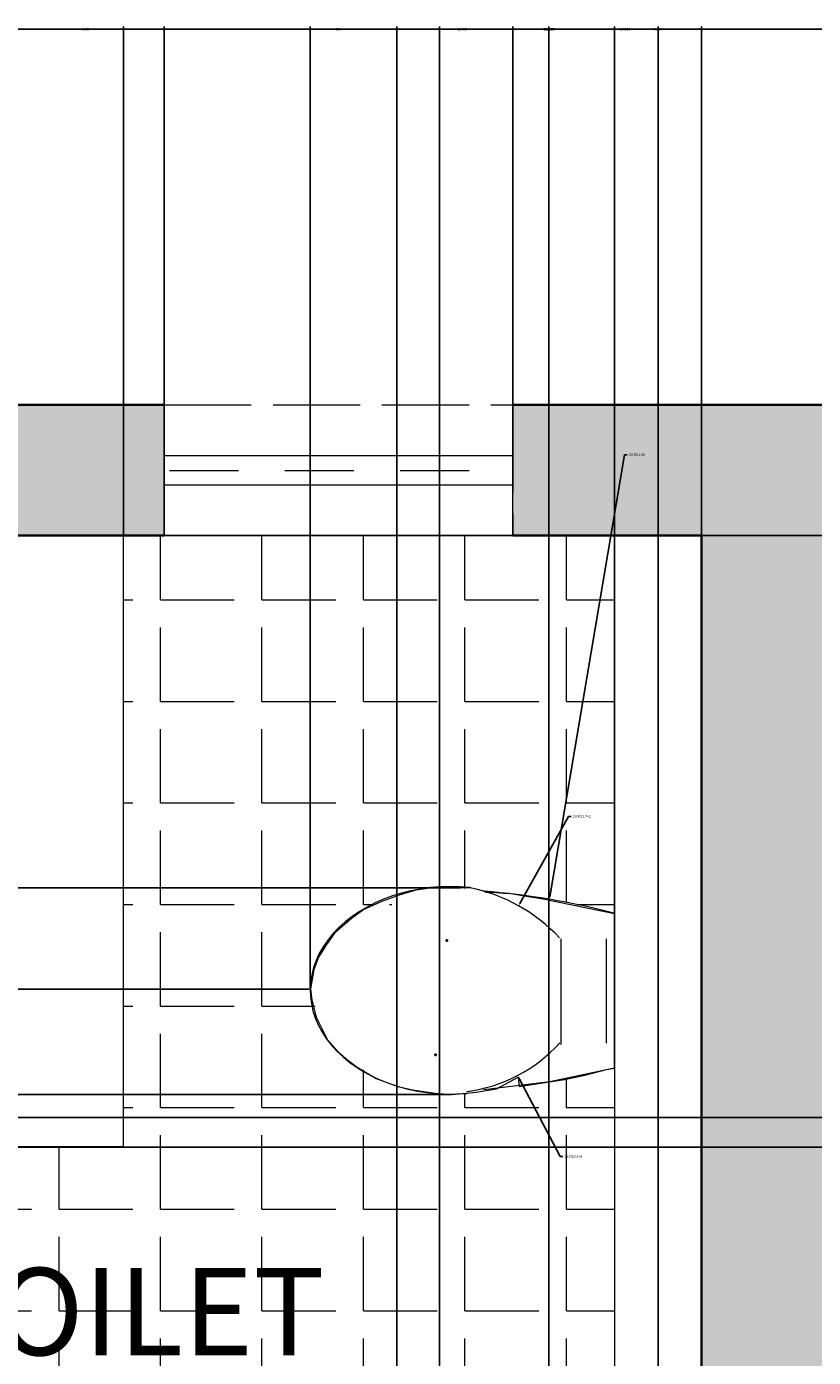
# Model space of a CAD drawing. Units: inches. Extents: x 6 to 575, y 34 to 566.
# Tile 11 of 21: x 151 to 205, y 474 to 566. Entities that reach past the tile are written whole.
import ezdxf

# ---------------------------------------------------------------- set-up
doc = ezdxf.new("R2010")
doc.units = ezdxf.units.IN
doc.linetypes.add('ACAD_ISO02W100', pattern=[15, 12, -3])
for name, color, linetype, lineweight in [('A-ANNO-DIMS', 2, 'Continuous', 18), ('A-AREA-IDEN', 6, 'Continuous', 20), ('A-FLOR-CASE', 2, 'Continuous', 18), ('A-FLOR-FIXT', 9, 'Continuous', 18), ('A-FLOR-PATT', 252, 'Continuous', 9), ('A-GLAZ-HIDN', 4, 'ACAD_ISO02W100', 18), ('A-GLAZ-PATT', 4, 'Continuous', 9), ('A-WALL-PATT', 251, 'Continuous', 9), ('WALLS', 7, 'Continuous', 35), ('WINDOWS', 4, 'Continuous', 20)]:
    doc.layers.add(name, color=color, linetype=linetype, lineweight=lineweight)
doc.styles.add('PDF Arial Narrow', font='txt')
doc.styles.get("Standard").update_dxf_attribs({"font": 'arial.ttf'})
doc.dimstyles.get("Standard").update_dxf_attribs({"dimtxt": 0.18, "dimasz": 0.18, "dimexe": 0.18, "dimexo": 0.0625, "dimgap": 0.09, "dimtad": 0, "dimtih": 1, "dimtoh": 1, "dimdec": 4, "dimzin": 0, "dimdsep": 46, "dimtxsty": 'Standard', "dimcen": 0.09, "dimadec": 0, "dimazin": 0, "dimtfac": 1, "dimtdec": 4, "dimtofl": 0, "dimtmove": 0, "dimatfit": 3, "dimfxl": 1, "dimtolj": 1, "dimtzin": 0, "dimarcsym": 0})

# ---------------------------------------------------------------- blocks, each defined once
blk = doc.blocks.new('*D30')
at = {"layer": 'A-ANNO-DIMS', "color": 0, "lineweight": -2, "transparency": 16777216}
for p, q in [((32.596, 539.801), (6.649, 539.801)), ((6.829, 539.621), (6.829, 299.97)), ((6.829, 59.955), (6.829, 299.606)), ((197.625, 59.775), (6.649, 59.775))]:
    blk.add_line(p, q, dxfattribs=at)
at = {"layer": 'A-ANNO-DIMS', "color": 0, "transparency": 16777216}
for points in [[(6.799, 539.621), (6.859, 539.621), (6.829, 539.801)], [(6.799, 59.955), (6.859, 59.955), (6.829, 59.775)]]:
    blk.add_solid(points, dxfattribs=at)
at = {"layer": 'Defpoints', "color": 0, "transparency": 16777216}
for p in [(32.659, 539.801), (6.829, 59.775), (197.687, 59.775)]:
    blk.add_point(p, dxfattribs=at)
at = {"layer": 'A-ANNO-DIMS', "color": 0, "transparency": 16777216, "insert": (6.829, 299.788), "char_height": 0.18, "attachment_point": 5}
blk.add_mtext('\\A1;480', dxfattribs=at)
blk = doc.blocks.new('*D31')
at = {"layer": 'A-ANNO-DIMS', "color": 0, "lineweight": -2, "transparency": 16777216}
for p, q in [((32.659, 539.863), (32.659, 565.811)), ((160.659, 539.863), (160.659, 565.811)), ((32.839, 565.631), (96.378, 565.631)), ((160.479, 565.631), (96.939, 565.631))]:
    blk.add_line(p, q, dxfattribs=at)
at = {"layer": 'A-ANNO-DIMS', "color": 0, "transparency": 16777216}
for points in [[(32.839, 565.661), (32.839, 565.601), (32.659, 565.631)], [(160.479, 565.661), (160.479, 565.601), (160.659, 565.631)]]:
    blk.add_solid(points, dxfattribs=at)
at = {"layer": 'Defpoints', "color": 0, "transparency": 16777216}
for p in [(160.659, 565.631), (32.659, 539.801), (160.659, 539.801)]:
    blk.add_point(p, dxfattribs=at)
at = {"layer": 'A-ANNO-DIMS', "color": 0, "transparency": 16777216, "insert": (96.659, 565.631), "char_height": 0.18, "attachment_point": 5}
blk.add_mtext('\\A1;128', dxfattribs=at)
blk = doc.blocks.new('*D32')
at = {"layer": 'A-ANNO-DIMS', "color": 0, "lineweight": -2, "transparency": 16777216}
for p, q in [((160.659, 539.863), (160.659, 565.811)), ((184.659, 539.863), (184.659, 565.811)), ((160.839, 565.631), (172.439, 565.631)), ((184.479, 565.631), (172.879, 565.631))]:
    blk.add_line(p, q, dxfattribs=at)
at = {"layer": 'A-ANNO-DIMS', "color": 0, "transparency": 16777216}
for points in [[(160.839, 565.661), (160.839, 565.601), (160.659, 565.631)], [(184.479, 565.661), (184.479, 565.601), (184.659, 565.631)]]:
    blk.add_solid(points, dxfattribs=at)
at = {"layer": 'Defpoints', "color": 0, "transparency": 16777216}
for p in [(184.659, 565.631), (160.659, 539.801), (184.659, 539.801)]:
    blk.add_point(p, dxfattribs=at)
at = {"layer": 'A-ANNO-DIMS', "color": 0, "transparency": 16777216, "insert": (172.659, 565.631), "char_height": 0.18, "attachment_point": 5}
blk.add_mtext('\\A1;24', dxfattribs=at)
blk = doc.blocks.new('*D33')
at = {"layer": 'A-ANNO-DIMS', "color": 0, "lineweight": -2, "transparency": 16777216}
for p, q in [((184.659, 539.863), (184.659, 565.811)), ((272.659, 539.863), (272.659, 565.811)), ((184.839, 565.631), (228.439, 565.631)), ((272.479, 565.631), (228.878, 565.631))]:
    blk.add_line(p, q, dxfattribs=at)
at = {"layer": 'A-ANNO-DIMS', "color": 0, "transparency": 16777216}
for points in [[(184.839, 565.661), (184.839, 565.601), (184.659, 565.631)], [(272.479, 565.661), (272.479, 565.601), (272.659, 565.631)]]:
    blk.add_solid(points, dxfattribs=at)
at = {"layer": 'Defpoints', "color": 0, "transparency": 16777216}
for p in [(272.659, 565.631), (184.659, 539.801), (272.659, 539.801)]:
    blk.add_point(p, dxfattribs=at)
at = {"layer": 'A-ANNO-DIMS', "color": 0, "transparency": 16777216, "insert": (228.659, 565.631), "char_height": 0.18, "attachment_point": 5}
blk.add_mtext('\\A1;88', dxfattribs=at)
blk = doc.blocks.new('*D68')
at = {"layer": 'A-ANNO-DIMS', "color": 0, "lineweight": -2, "transparency": 16777216}
for p, q in [((206.596, 530.801), (6.649, 530.801)), ((6.829, 530.621), (6.829, 509.957)), ((6.829, 488.928), (6.829, 509.593)), ((248.571, 488.748), (6.649, 488.748))]:
    blk.add_line(p, q, dxfattribs=at)
at = {"layer": 'A-ANNO-DIMS', "color": 0, "transparency": 16777216}
for points in [[(6.799, 530.621), (6.859, 530.621), (6.829, 530.801)], [(6.799, 488.928), (6.859, 488.928), (6.829, 488.748)]]:
    blk.add_solid(points, dxfattribs=at)
at = {"layer": 'Defpoints', "color": 0, "transparency": 16777216}
for p in [(206.659, 530.801), (6.829, 488.748), (248.633, 488.748)]:
    blk.add_point(p, dxfattribs=at)
at = {"layer": 'A-ANNO-DIMS', "color": 0, "transparency": 16777216, "insert": (6.829, 509.775), "char_height": 0.18, "attachment_point": 5}
blk.add_mtext('\\A1;42.05', dxfattribs=at)
blk = doc.blocks.new('*D71')
at = {"layer": 'A-ANNO-DIMS', "color": 0, "lineweight": -2, "transparency": 16777216}
for p, q in [((246.62, 490.777), (6.649, 490.777)), ((6.829, 490.597), (6.829, 489.945)), ((6.829, 488.928), (6.829, 489.581)), ((248.571, 488.748), (6.649, 488.748))]:
    blk.add_line(p, q, dxfattribs=at)
at = {"layer": 'A-ANNO-DIMS', "color": 0, "transparency": 16777216}
for points in [[(6.799, 490.597), (6.859, 490.597), (6.829, 490.777)], [(6.799, 488.928), (6.859, 488.928), (6.829, 488.748)]]:
    blk.add_solid(points, dxfattribs=at)
at = {"layer": 'Defpoints', "color": 0, "transparency": 16777216}
for p in [(246.683, 490.777), (6.829, 488.748), (248.633, 488.748)]:
    blk.add_point(p, dxfattribs=at)
at = {"layer": 'A-ANNO-DIMS', "color": 0, "transparency": 16777216, "insert": (6.829, 489.763), "char_height": 0.18, "attachment_point": 5}
blk.add_mtext('\\A1;2.03', dxfattribs=at)
blk = doc.blocks.new('*D109')
at = {"layer": 'A-ANNO-DIMS', "color": 0, "lineweight": -2, "transparency": 16777216}
for p, q in [((112.851, 431.863), (112.851, 565.811)), ((197.659, 431.863), (197.659, 565.811)), ((113.031, 565.631), (154.931, 565.631)), ((197.479, 565.631), (155.579, 565.631))]:
    blk.add_line(p, q, dxfattribs=at)
at = {"layer": 'A-ANNO-DIMS', "color": 0, "transparency": 16777216}
for points in [[(113.031, 565.661), (113.031, 565.601), (112.851, 565.631)], [(197.479, 565.661), (197.479, 565.601), (197.659, 565.631)]]:
    blk.add_solid(points, dxfattribs=at)
at = {"layer": 'Defpoints', "color": 0, "transparency": 16777216}
for p in [(197.659, 565.631), (112.851, 431.801), (197.659, 431.801)]:
    blk.add_point(p, dxfattribs=at)
at = {"layer": 'A-ANNO-DIMS', "color": 0, "transparency": 16777216, "insert": (155.255, 565.631), "char_height": 0.18, "attachment_point": 5}
blk.add_mtext('\\A1;84.8', dxfattribs=at)
blk = doc.blocks.new('*D175')
at = {"layer": 'A-ANNO-DIMS', "color": 0, "lineweight": -2, "transparency": 16777216}
for p, q in [((121.659, 530.863), (121.659, 565.811)), ((157.869, 530.898), (157.869, 565.811)), ((121.839, 565.631), (139.387, 565.631)), ((157.689, 565.631), (140.14, 565.631))]:
    blk.add_line(p, q, dxfattribs=at)
at = {"layer": 'A-ANNO-DIMS', "color": 0, "transparency": 16777216}
for points in [[(121.839, 565.661), (121.839, 565.601), (121.659, 565.631)], [(157.689, 565.661), (157.689, 565.601), (157.869, 565.631)]]:
    blk.add_solid(points, dxfattribs=at)
at = {"layer": 'Defpoints', "color": 0, "transparency": 16777216}
for p in [(157.869, 565.631), (121.659, 530.801), (157.869, 530.836)]:
    blk.add_point(p, dxfattribs=at)
at = {"layer": 'A-ANNO-DIMS', "color": 0, "transparency": 16777216, "insert": (139.764, 565.631), "char_height": 0.18, "attachment_point": 5}
blk.add_mtext('\\A1;36.21', dxfattribs=at)
blk = doc.blocks.new('*D181')
at = {"layer": 'A-ANNO-DIMS', "color": 0, "lineweight": -2, "transparency": 16777216}
for p, q in [((197.596, 530.801), (6.649, 530.801)), ((6.829, 530.621), (6.829, 515.387)), ((6.829, 499.788), (6.829, 515.023)), ((170.657, 499.608), (6.649, 499.608))]:
    blk.add_line(p, q, dxfattribs=at)
at = {"layer": 'A-ANNO-DIMS', "color": 0, "transparency": 16777216}
for points in [[(6.799, 530.621), (6.859, 530.621), (6.829, 530.801)], [(6.799, 499.788), (6.859, 499.788), (6.829, 499.608)]]:
    blk.add_solid(points, dxfattribs=at)
at = {"layer": 'Defpoints', "color": 0, "transparency": 16777216}
for p in [(197.659, 530.801), (6.829, 499.608), (170.719, 499.608)]:
    blk.add_point(p, dxfattribs=at)
at = {"layer": 'A-ANNO-DIMS', "color": 0, "transparency": 16777216, "insert": (6.829, 515.205), "char_height": 0.18, "attachment_point": 5}
blk.add_mtext('\\A1;31.19', dxfattribs=at)
blk = doc.blocks.new('*D182')
at = {"layer": 'A-ANNO-DIMS', "color": 0, "lineweight": -2, "transparency": 16777216}
for p, q in [((170.719, 499.671), (170.719, 565.811)), ((191.651, 504.84), (191.651, 565.811)), ((170.899, 565.631), (180.79, 565.631)), ((191.471, 565.631), (181.581, 565.631))]:
    blk.add_line(p, q, dxfattribs=at)
at = {"layer": 'A-ANNO-DIMS', "color": 0, "transparency": 16777216}
for points in [[(170.899, 565.661), (170.899, 565.601), (170.719, 565.631)], [(191.471, 565.661), (191.471, 565.601), (191.651, 565.631)]]:
    blk.add_solid(points, dxfattribs=at)
at = {"layer": 'Defpoints', "color": 0, "transparency": 16777216}
for p in [(191.651, 565.631), (191.651, 504.777), (170.719, 499.608)]:
    blk.add_point(p, dxfattribs=at)
at = {"layer": 'A-ANNO-DIMS', "color": 0, "transparency": 16777216, "insert": (181.185, 565.631), "char_height": 0.18, "attachment_point": 5}
blk.add_mtext('\\A1;20.93', dxfattribs=at)
blk = doc.blocks.new('*D183')
at = {"layer": 'A-ANNO-DIMS', "color": 0, "lineweight": -2, "transparency": 16777216}
for p, q in [((181.056, 506.572), (6.649, 506.572)), ((6.829, 506.392), (6.829, 499.652)), ((6.829, 492.552), (6.829, 499.291)), ((180.432, 492.372), (6.649, 492.372))]:
    blk.add_line(p, q, dxfattribs=at)
at = {"layer": 'A-ANNO-DIMS', "color": 0, "transparency": 16777216}
for points in [[(6.799, 506.392), (6.859, 506.392), (6.829, 506.572)], [(6.799, 492.552), (6.859, 492.552), (6.829, 492.372)]]:
    blk.add_solid(points, dxfattribs=at)
at = {"layer": 'Defpoints', "color": 0, "transparency": 16777216}
for p in [(6.829, 506.572), (181.118, 506.572), (180.494, 492.372)]:
    blk.add_point(p, dxfattribs=at)
at = {"layer": 'A-ANNO-DIMS', "color": 0, "transparency": 16777216, "insert": (6.829, 499.472), "char_height": 0.18, "attachment_point": 5}
blk.add_mtext('\\A1;14.2', dxfattribs=at)
blk = doc.blocks.new('*D184')
at = {"layer": 'A-ANNO-DIMS', "color": 0, "lineweight": -2, "transparency": 16777216}
for p, q in [((191.651, 504.84), (191.651, 565.811)), ((197.659, 530.863), (197.659, 565.811)), ((191.831, 565.631), (194.261, 565.631)), ((197.479, 565.631), (195.049, 565.631))]:
    blk.add_line(p, q, dxfattribs=at)
at = {"layer": 'A-ANNO-DIMS', "color": 0, "transparency": 16777216}
for points in [[(191.831, 565.661), (191.831, 565.601), (191.651, 565.631)], [(197.479, 565.661), (197.479, 565.601), (197.659, 565.631)]]:
    blk.add_solid(points, dxfattribs=at)
at = {"layer": 'Defpoints', "color": 0, "transparency": 16777216}
for p in [(197.659, 565.631), (197.659, 530.801), (191.651, 504.777)]:
    blk.add_point(p, dxfattribs=at)
at = {"layer": 'A-ANNO-DIMS', "color": 0, "transparency": 16777216, "insert": (194.655, 565.631), "char_height": 0.18, "attachment_point": 5}
blk.add_mtext('\\A1;6.008', dxfattribs=at)
blk = doc.blocks.new('*D185')
at = {"layer": 'A-ANNO-DIMS', "color": 0, "lineweight": -2, "transparency": 16777216}
for p, q in [((176.671, 440.863), (176.671, 565.811)), ((197.659, 470.901), (197.659, 565.811)), ((176.851, 565.631), (186.7, 565.631)), ((197.479, 565.631), (187.63, 565.631))]:
    blk.add_line(p, q, dxfattribs=at)
at = {"layer": 'A-ANNO-DIMS', "color": 0, "transparency": 16777216}
for points in [[(176.851, 565.661), (176.851, 565.601), (176.671, 565.631)], [(197.479, 565.661), (197.479, 565.601), (197.659, 565.631)]]:
    blk.add_solid(points, dxfattribs=at)
at = {"layer": 'Defpoints', "color": 0, "transparency": 16777216}
for p in [(197.659, 565.631), (197.659, 470.839), (176.671, 440.801)]:
    blk.add_point(p, dxfattribs=at)
at = {"layer": 'A-ANNO-DIMS', "color": 0, "transparency": 16777216, "insert": (187.165, 565.631), "char_height": 0.18, "attachment_point": 5}
blk.add_mtext('\\A1;20.987', dxfattribs=at)
blk = doc.blocks.new('*D187')
at = {"layer": 'A-ANNO-DIMS', "color": 0, "lineweight": -2, "transparency": 16777216}
for p, q in [((179.613, 456.49), (179.613, 565.811)), ((194.671, 456.402), (194.671, 565.811)), ((179.793, 565.631), (186.687, 565.631)), ((194.491, 565.631), (187.598, 565.631))]:
    blk.add_line(p, q, dxfattribs=at)
at = {"layer": 'A-ANNO-DIMS', "color": 0, "transparency": 16777216}
for points in [[(179.793, 565.661), (179.793, 565.601), (179.613, 565.631)], [(194.491, 565.661), (194.491, 565.601), (194.671, 565.631)]]:
    blk.add_solid(points, dxfattribs=at)
at = {"layer": 'Defpoints', "color": 0, "transparency": 16777216}
for p in [(194.671, 565.631), (179.613, 456.427), (194.671, 456.339)]:
    blk.add_point(p, dxfattribs=at)
at = {"layer": 'A-ANNO-DIMS', "color": 0, "transparency": 16777216, "insert": (187.142, 565.631), "char_height": 0.18, "attachment_point": 5}
blk.add_mtext('\\A1;15.058', dxfattribs=at)
blk = doc.blocks.new('*D190')
at = {"layer": 'A-ANNO-DIMS', "color": 0, "lineweight": -2, "transparency": 16777216}
for p, q in [((187.142, 456.446), (187.142, 565.811)), ((197.659, 440.863), (197.659, 565.811)), ((187.322, 565.631), (191.945, 565.631)), ((197.479, 565.631), (192.856, 565.631))]:
    blk.add_line(p, q, dxfattribs=at)
at = {"layer": 'A-ANNO-DIMS', "color": 0, "transparency": 16777216}
for points in [[(187.322, 565.661), (187.322, 565.601), (187.142, 565.631)], [(197.479, 565.661), (197.479, 565.601), (197.659, 565.631)]]:
    blk.add_solid(points, dxfattribs=at)
at = {"layer": 'Defpoints', "color": 0, "transparency": 16777216}
for p in [(187.142, 565.631), (187.142, 456.383), (197.659, 440.801)]:
    blk.add_point(p, dxfattribs=at)
at = {"layer": 'A-ANNO-DIMS', "color": 0, "transparency": 16777216, "insert": (192.4, 565.631), "char_height": 0.18, "attachment_point": 5}
blk.add_mtext('\\A1;10.516', dxfattribs=at)
blk = doc.blocks.new('*D226')
at = {"layer": 'A-ANNO-DIMS', "color": 0, "lineweight": -2, "transparency": 16777216}
for p, q in [((192.35, 536.366), (187.209, 505.964)), ((192.53, 536.366), (192.35, 536.366)), ((178.56, 454.733), (178.56, 454.913)), ((178.47, 454.823), (178.65, 454.823))]:
    blk.add_line(p, q, dxfattribs=at)
at = {"layer": 'A-ANNO-DIMS', "color": 0, "transparency": 16777216}
blk.add_solid([(187.179, 505.969), (187.239, 505.959), (187.179, 505.787)], dxfattribs=at)
at = {"layer": 'Defpoints', "color": 0, "transparency": 16777216}
for p in [(187.179, 505.787), (178.56, 454.823)]:
    blk.add_point(p, dxfattribs=at)
at = {"layer": 'A-ANNO-DIMS', "color": 0, "transparency": 16777216, "insert": (193.205, 536.366), "char_height": 0.18, "attachment_point": 5}
blk.add_mtext('\\A1;2X R51.69', dxfattribs=at)
blk = doc.blocks.new('*D235')
at = {"layer": 'A-ANNO-DIMS', "color": 0, "lineweight": -2, "transparency": 16777216}
for p, q in [((188.495, 511.488), (185.15, 505.493)), ((188.675, 511.488), (188.495, 511.488)), ((179.25, 495.082), (179.43, 495.082)), ((179.34, 494.992), (179.34, 495.172))]:
    blk.add_line(p, q, dxfattribs=at)
at = {"layer": 'A-ANNO-DIMS', "color": 0, "transparency": 16777216}
blk.add_solid([(185.123, 505.508), (185.176, 505.478), (185.062, 505.336)], dxfattribs=at)
at = {"layer": 'Defpoints', "color": 0, "transparency": 16777216}
for p in [(185.062, 505.336), (179.34, 495.082)]:
    blk.add_point(p, dxfattribs=at)
at = {"layer": 'A-ANNO-DIMS', "color": 0, "transparency": 16777216, "insert": (189.419, 511.488), "char_height": 0.18, "attachment_point": 5}
blk.add_mtext('\\A1;2X R11.742', dxfattribs=at)
blk = doc.blocks.new('*D238')
at = {"layer": 'A-ANNO-DIMS', "color": 0, "lineweight": -2, "transparency": 16777216}
for p, q in [((180.03, 502.963), (180.21, 502.963)), ((180.12, 502.873), (180.12, 503.053)), ((187.915, 488.092), (185.076, 493.509)), ((188.095, 488.092), (187.915, 488.092))]:
    blk.add_line(p, q, dxfattribs=at)
at = {"layer": 'A-ANNO-DIMS', "color": 0, "transparency": 16777216}
blk.add_solid([(185.102, 493.523), (185.049, 493.495), (184.992, 493.669)], dxfattribs=at)
at = {"layer": 'Defpoints', "color": 0, "transparency": 16777216}
for p in [(180.12, 502.963), (184.992, 493.669)]:
    blk.add_point(p, dxfattribs=at)
at = {"layer": 'A-ANNO-DIMS', "color": 0, "transparency": 16777216, "insert": (188.84, 488.092), "char_height": 0.18, "attachment_point": 5}
blk.add_mtext('\\A1;2X R10.494', dxfattribs=at)

msp = doc.modelspace()

# ---------------------------------------------------------------- hatches: boundary and pattern name
at = {"layer": 'A-FLOR-PATT'}
h = msp.add_hatch(dxfattribs=at)
h.set_pattern_fill('ANGLE', color=256)
h.set_pattern_definition([(0, (-98.035, 170.1465), (0, 6.985), [5.08, -1.905]), (90, (-98.035, 170.1465), (-6.985, 4e-16), [5.08, -1.905])])
edge = h.paths.add_edge_path()
edge.add_line((191.6511, 494.1664), (190.4028, 493.9036))
edge.add_line((190.4028, 493.9036), (189.6226, 493.6983))
edge.add_line((189.6226, 493.6983), (188.2183, 493.3862))
edge.add_line((188.2183, 493.3862), (187.2685, 493.2437))
edge.add_line((187.2685, 493.2437), (187.204, 493.2302))
edge.add_line((187.204, 493.2302), (187.0709, 493.2141))
edge.add_line((187.0709, 493.2141), (185.0975, 492.9181))
edge.add_line((185.0975, 492.9181), (185.0904, 492.9751))
edge.add_line((185.0904, 492.9751), (183.6001, 492.7952))
edge.add_line((183.6001, 492.7952), (183.5371, 492.7621))
edge.add_line((183.5371, 492.7621), (181.5041, 492.4232))
edge.add_spline(control_points=[(181.5178, 492.4356), (181.2536, 492.4138), (180.9898, 492.4), (180.727, 492.3941)], knot_values=[2.9292163, 2.9292163, 2.9292163, 2.9292163, 3, 3, 3, 3], degree=3, periodic=0)
edge.add_line((180.727, 492.3941), (180.4943, 492.372))
edge.add_line((180.4943, 492.372), (180.175, 492.3932))
edge.add_spline(control_points=[(180.175, 492.3932), (179.0187, 492.4156), (177.8901, 492.5895), (176.8377, 492.8977)], knot_values=[2.5659353, 2.5659353, 2.5659353, 2.5659353, 2.8794912, 2.8794912, 2.8794912, 2.8794912], degree=3, periodic=0)
edge.add_line((176.8377, 492.8977), (176.5264, 492.9696))
edge.add_spline(control_points=[(176.656, 492.9525), (176.2658, 493.0735), (175.8866, 493.2132), (175.521, 493.3707)], knot_values=[2.4305318, 2.4305318, 2.4305318, 2.4305318, 2.5478122, 2.5478122, 2.5478122, 2.5478122], degree=3, periodic=0)
edge.add_line((175.521, 493.3707), (175.267, 493.4642))
edge.add_line((175.267, 493.4642), (175.098, 493.5637))
edge.add_spline(control_points=[(175.098, 493.5637), (173.9351, 494.1251), (172.9292, 494.8734), (172.1696, 495.7766)], knot_values=[2, 2, 2, 2, 2.3846171, 2.3846171, 2.3846171, 2.3846171], degree=3, periodic=0)
edge.add_line((172.9656, 494.9581), (172.8363, 495.1004))
edge.add_spline(control_points=[(175.098, 493.5637), (173.9351, 494.1251), (172.9292, 494.8734), (172.1696, 495.7766)], knot_values=[2, 2, 2, 2, 2.3846171, 2.3846171, 2.3846171, 2.3846171], degree=3, periodic=0)
edge.add_line((171.9925, 495.9563), (171.8762, 496.1888))
edge.add_spline(control_points=[(172.1696, 495.7766), (170.1947, 498.1251), (170.2393, 501.0999), (172.2842, 503.4158)], knot_values=[1, 1, 1, 1, 2, 2, 2, 2], degree=3, periodic=0)
edge.add_line((170.6556, 499.1388), (170.6881, 499.323))
edge.add_spline(control_points=[(172.1696, 495.7766), (170.1947, 498.1251), (170.2393, 501.0999), (172.2842, 503.4158)], knot_values=[1, 1, 1, 1, 2, 2, 2, 2], degree=3, periodic=0)
edge.add_spline(control_points=[(172.2842, 503.4158), (174.3291, 505.7317), (178.0076, 506.9734), (181.7304, 506.6045)], knot_values=[0, 0, 0, 0, 1, 1, 1, 1], degree=3, periodic=0)
edge.add_line((174.0548, 504.9343), (174.2554, 505.022))
edge.add_spline(control_points=[(172.2842, 503.4158), (174.3291, 505.7317), (178.0076, 506.9734), (181.7304, 506.6045)], knot_values=[0, 0, 0, 0, 1, 1, 1, 1], degree=3, periodic=0)
edge.add_line((178.4031, 506.5313), (178.1947, 506.4718))
edge.add_spline(control_points=[(172.2842, 503.4158), (174.3291, 505.7317), (178.0076, 506.9734), (181.7304, 506.6045)], knot_values=[0, 0, 0, 0, 1, 1, 1, 1], degree=3, periodic=0)
edge.add_line((181.5796, 506.6123), (181.6459, 506.5957))
edge.add_arc((179.34, 495.0824), 11.742, 73.636084, 78.674278, ccw=False)
edge.add_arc((178.5598, 454.8227), 51.688, 83.52982, 85.463383, ccw=False)
edge.add_line((184.3843, 506.1814), (184.5513, 506.1814))
edge.add_line((184.5513, 506.1814), (184.7887, 506.134))
edge.add_arc((178.5598, 454.8227), 51.688, 75.328548, 83.07845, ccw=False)
edge.add_line((191.6511, 504.8253), (191.6511, 530.801))
edge.add_line((191.6511, 530.801), (184.6586, 530.801))
edge.add_line((184.6586, 530.801), (160.6586, 530.801))
edge.add_line((160.6586, 530.801), (157.8686, 530.801))
edge.add_line((157.8686, 530.801), (157.8686, 488.7831))
edge.add_line((157.8686, 488.7831), (121.6586, 488.7831))
edge.add_line((121.6586, 488.7831), (121.6586, 474.801))
edge.add_line((121.6586, 474.801), (120.6068, 474.801))
edge.add_line((120.6068, 474.801), (120.6068, 474.0666))
edge.add_arc((120.0902, 447.538), 26.5336, 62.388015, 88.884314, ccw=False)
edge.add_line((132.388, 471.0496), (132.3995, 471.0696))
edge.add_line((132.3995, 471.0696), (133.357, 470.5168))
edge.add_line((133.357, 470.5168), (120.0902, 447.538))
edge.add_line((120.0902, 447.538), (120.6068, 447.538))
edge.add_line((120.6068, 447.538), (121.6586, 446.801))
edge.add_line((121.6586, 446.801), (121.6586, 440.801))
edge.add_line((121.6586, 440.801), (176.6714, 440.801))
edge.add_line((176.6714, 440.801), (176.6714, 470.8385))
edge.add_line((176.6714, 470.8385), (191.6511, 470.8385))
edge.add_line((191.6511, 470.8385), (191.6511, 494.1664))
h = msp.add_hatch(dxfattribs=at)
h.set_pattern_fill('BRICK', color=256)
h.set_pattern_definition([(0, (-98.035, 170.1465), (0, 6.35), []), (90, (-98.035, 170.147), (-12.7, 8e-16), [6.35, -6.35]), (90, (-91.685, 170.147), (-12.7, 8e-16), [-6.35, 6.35])])
h.paths.add_polyline_path([(180.8711, 269.7588), (182.4439, 270.6668), (182.4628, 270.6341, -0.1161983), (201.8275, 275.5902), (201.8275, 276.801), (197.6586, 276.801), (197.6586, 293.1641), (182.6401, 293.1641), (182.6401, 348.324), (197.6586, 348.324), (197.6586, 407.7709), (112.8513, 407.7709), (112.8513, 431.801), (111.6586, 431.801), (111.6586, 440.801), (117.6586, 440.801), (117.6586, 446.801), (117.6586, 448.2751), (117.6586, 473.3269), (117.6586, 474.801), (117.6586, 515.5941), (100.2533, 515.5941, -1), (83.0548, 515.5941), (65.6494, 515.5941), (65.6494, 440.801), (82.8918, 440.801), (82.8918, 431.801), (82.8918, 407.7709), (41.6586, 407.7709), (41.6586, 379.0637), (62.6459, 379.0637), (62.6459, 358.0764), (122.565, 358.0764), (122.565, 286.0643), (62.6459, 286.0643), (62.6459, 265.077), (41.6586, 265.077), (41.6586, 224.801), (41.6586, 212.801), (71.6586, 212.801), (167.6586, 212.801), (197.6586, 212.801), (197.6586, 230.801), (201.8157, 230.801), (201.8157, 233.4817)])
h.paths.add_polyline_path([(133.3414, 245.1275), (133.3317, 245.1352), (133.3317, 245.104)], flags=16)
h.paths.add_polyline_path([(133.3317, 222.1662), (85.3496, 222.1662), (85.3496, 243.7443, -0.5009073), (87.1831, 246.1963), (107.4292, 246.1963), (111.2522, 246.1963), (131.4202, 246.1963, -0.4142136), (133.3317, 244.2848)], flags=16)
h.paths.add_polyline_path([(72.7105, 244.4018), (72.7105, 220.3718), (48.6804, 220.3718), (48.6804, 244.4018)], flags=16)
h.paths.add_polyline_path([(71.7466, 237.8955, -1), (59.8096, 237.8955, -1)], flags=0)
at = {"layer": 'A-GLAZ-PATT'}
h = msp.add_hatch(dxfattribs=at)
h.set_pattern_fill('CLAY', color=256)
h.set_pattern_definition([(0, (-85.0353, 170.1465), (0, 4.7625), []), (0, (-85.0353, 170.9403), (0, 4.7625), []), (0, (-85.0353, 171.734), (0, 4.7625), []), (0, (-85.0353, 173.3215), (0, 4.7625), [4.7625, -3.175])])
h.paths.add_polyline_path([(160.6586, 536.301), (160.6586, 534.301), (184.6586, 534.301), (184.6586, 536.301)])
at = {"layer": 'A-WALL-PATT'}
h = msp.add_hatch(color=256, dxfattribs=at)
h.dxf.hatch_style = 1
h.paths.add_polyline_path([(160.6586, 539.801), (32.6586, 539.801), (32.6586, 272.801), (41.6586, 272.801), (41.6586, 286.0643), (41.6586, 358.0764), (41.6586, 379.0637), (41.6586, 407.7709), (41.6194, 407.7709), (41.6194, 431.801), (82.8918, 431.801), (82.8918, 440.801), (65.6494, 440.801), (65.6494, 440.7732), (41.6194, 440.7732), (41.6194, 515.5941), (41.6586, 530.801), (117.6586, 530.801), (117.6586, 474.801), (120.6068, 474.801), (121.6586, 474.801), (121.6586, 530.801), (137.4275, 530.801), (137.4275, 530.8356), (141.2505, 530.8356), (160.6586, 530.801)])
h.paths.add_polyline_path([(71.6586, 212.801), (41.6586, 212.801), (41.6586, 224.801), (32.6586, 224.801), (32.6586, 203.801), (71.6586, 203.801)])
h.paths.add_polyline_path([(206.6586, 215.801), (246.6586, 215.801), (246.6586, 224.801), (206.6586, 224.801), (206.6586, 230.801), (201.8157, 230.801), (197.6586, 230.801), (197.6586, 212.801), (167.6586, 212.801), (167.6586, 203.801), (206.6586, 203.801)])
h.paths.add_polyline_path([(383.6586, 224.801), (334.6586, 224.801), (334.6586, 215.801), (374.6586, 215.801), (374.6586, 203.801), (384.0753, 203.801), (407.6586, 203.801), (407.6586, 212.801), (383.6586, 212.801)])
h.paths.add_polyline_path([(548.6586, 270.801), (539.6586, 270.801), (539.6586, 212.801), (515.6586, 212.801), (515.6586, 203.801), (548.6586, 203.801)])
h.paths.add_polyline_path([(548.6586, 412.801), (545.7108, 412.801), (539.6586, 412.801), (539.6586, 382.801), (433.708, 382.801), (433.708, 378.801), (539.6586, 378.801), (539.6586, 366.801), (548.6586, 366.801)])
h.paths.add_polyline_path([(548.6586, 539.801), (455.9436, 539.801), (455.9436, 530.801), (539.6586, 530.801), (539.6586, 440.801), (548.6586, 440.801)])
h.paths.add_polyline_path([(407.9436, 539.801), (362.6586, 539.801), (362.6586, 530.801), (374.6586, 530.801), (374.6586, 452.801), (354.6586, 452.801), (354.6586, 448.801), (374.6586, 448.801), (374.6586, 278.801), (383.6586, 278.801), (383.6586, 530.801), (407.9436, 530.801)])
h.paths.add_polyline_path([(338.6586, 539.801), (320.6586, 539.801), (320.6586, 530.801), (322.6586, 530.801), (322.6586, 448.801), (326.6586, 448.801), (326.6586, 530.801), (338.6586, 530.801)])
h.paths.add_polyline_path([(272.6586, 539.801), (184.6586, 539.801), (184.6586, 530.801), (197.6586, 530.801), (197.6586, 440.801), (176.6714, 440.801), (121.6586, 440.801), (121.6586, 446.801), (117.6586, 446.801), (117.6586, 440.801), (111.6586, 440.801), (111.6586, 431.801), (197.6586, 431.801), (197.6586, 407.7709), (197.6586, 276.801), (206.6586, 276.801), (206.6586, 530.801), (272.6586, 530.801)])

# ---------------------------------------------------------------- linework, layer by layer
at = {"layer": 'A-FLOR-CASE'}
msp.add_lwpolyline([(191.6511, 530.8356), (191.6511, 470.8385)], dxfattribs=at)
at = {"layer": 'A-FLOR-FIXT'}
for points in [[(121.9016, 488.7831), (157.8686, 488.7831), (157.8686, 530.8356)], [(191.6511, 504.7771), (191.6511, 494.1664), (187.204, 493.2302), (182.6789, 492.684)], [(187.9842, 495.8048), (187.9842, 503.0606)], [(191.105, 495.8828), (191.105, 503.0606)]]:
    msp.add_lwpolyline(points, dxfattribs=at)
msp.add_lwpolyline([(191.6511, 504.7771), (186.7359, 505.7913), (185.3315, 506.0254), (184.9414, 506.1034), (184.3953, 506.1814), (184.0052, 506.1814), (183.303, 506.2594), (183.147, 506.2594), (182.9129, 506.2594), (182.8349, 506.2594), (182.6789, 506.3375), (181.7426, 506.5715), (181.1185, 506.5715), (179.168, 506.5715), (177.9977, 506.4155), (176.9054, 506.1034), (175.6571, 505.6353), (174.4088, 505.0892), (173.5506, 504.465), (172.3803, 503.4507), (171.8341, 502.6705), (171.288, 501.8123), (170.9759, 500.9541), (170.7419, 499.6278), (170.8199, 498.8476), (171.132, 497.6773), (171.9122, 496.1169), (172.6924, 495.2587), (173.3165, 494.7125), (173.9407, 494.2444), (175.267, 493.4642), (176.7494, 492.9181), (177.7636, 492.684), (179.324, 492.45), (180.4943, 492.372), (182.1327, 492.528), (183.5371, 492.7621), (185.0195, 493.5423), (185.0975, 492.9181), (188.2183, 493.3862), (189.6226, 493.6983), (191.105, 494.0884), (191.6511, 494.1664)], close=True, dxfattribs=at)
for centre, radius, start, end in [((179.34, 495.0824), 11.742, 43.291631, 78.376459), ((178.5598, 454.8227), 51.688, 75.377215, 85.424212), ((180.1202, 502.9627), 10.4936, 277.52563, 317.801513)]:
    msp.add_arc(centre, radius, start, end, dxfattribs=at)
msp.add_open_spline([(181.7304, 506.6045), (178.0076, 506.9734), (174.3291, 505.7317), (172.2842, 503.4158), (170.2393, 501.0999), (170.1947, 498.1251), (172.1696, 495.7766), (174.1445, 493.4282), (177.7848, 492.1271), (181.5178, 492.4356)], degree=3, knots=[0, 0, 0, 0, 1, 1, 1, 2, 2, 2, 3, 3, 3, 3], dxfattribs=at)
at = {"layer": 'A-GLAZ-HIDN', "ltscale": 0.5}
msp.add_lwpolyline([(160.6586, 539.801), (184.6586, 539.801), (184.6586, 530.801), (160.6586, 530.801)], close=True, dxfattribs=at)
at = {"layer": 'WALLS'}
for p, q in [((32.6586, 539.801), (160.6586, 539.801)), ((184.6586, 539.801), (272.6586, 539.801)), ((121.6586, 530.801), (160.6586, 530.801)), ((184.6586, 530.801), (197.6586, 530.801)), ((197.6586, 440.801), (197.6586, 530.801))]:
    msp.add_line(p, q, dxfattribs=at)
at = {"layer": 'WINDOWS'}
for p, q in [((160.6586, 530.801), (160.6586, 539.801)), ((160.6586, 539.801), (160.6586, 530.801)), ((184.6586, 530.801), (184.6586, 539.801)), ((160.6586, 536.301), (184.6586, 536.301)), ((160.6586, 534.301), (184.6586, 534.301))]:
    msp.add_line(p, q, dxfattribs=at)

# ---------------------------------------------------------------- texts
at = {"layer": 'A-AREA-IDEN', "insert": (144.1573, 476.6524), "char_height": 6.0005, "attachment_point": 4, "style": 'PDF Arial Narrow'}
msp.add_mtext('TOILET', dxfattribs=at)

# ---------------------------------------------------------------- dimensions: what is measured, and where the dimension line sits
at = {"layer": 'A-ANNO-DIMS'}
for base, p1, p2, override, picture, middle in [((160.6586, 565.631), (32.6586, 539.801), (160.6586, 539.801), {"dimdec": 0, "dimlfac": 1, "dimrnd": 0, "dimzin": 0, "dimdsep": 46, "dimlunit": 2}, '*D31', (96.6586, 565.631)), ((197.6586, 565.631), (112.8513, 431.801), (197.6586, 431.801), {"dimdec": 1, "dimlfac": 1, "dimrnd": 0, "dimzin": 0, "dimdsep": 46, "dimlunit": 2}, '*D109', (155.255, 565.631)), ((157.8686, 565.631), (121.6586, 530.801), (157.8686, 530.8356), {"dimdec": 2, "dimlfac": 1, "dimrnd": 0, "dimzin": 0, "dimdsep": 46, "dimlunit": 2}, '*D175', (139.7636, 565.631)), ((184.6586, 565.631), (160.6586, 539.801), (184.6586, 539.801), {"dimdec": 0, "dimlfac": 1, "dimrnd": 0, "dimzin": 0, "dimdsep": 46, "dimlunit": 2}, '*D32', (172.6586, 565.631)), ((191.6511, 565.631), (170.7195, 499.6084), (191.6511, 504.7771), {"dimdec": 2, "dimlfac": 1, "dimrnd": 0, "dimzin": 0, "dimdsep": 46, "dimlunit": 2}, '*D182', (181.1853, 565.631)), ((197.6586, 565.631), (176.6714, 440.801), (197.6586, 470.8385), {"dimdec": 3, "dimlfac": 1, "dimrnd": 0, "dimzin": 0, "dimdsep": 46, "dimlunit": 2}, '*D185', (187.165, 565.631)), ((194.6712, 565.631), (179.6134, 456.4271), (194.6712, 456.339), {"dimdec": 3, "dimlfac": 1, "dimrnd": 0, "dimzin": 0, "dimdsep": 46, "dimlunit": 2}, '*D187', (187.1423, 565.631)), ((272.6586, 565.631), (184.6586, 539.801), (272.6586, 539.801), {"dimdec": 0, "dimlfac": 1, "dimrnd": 0, "dimzin": 0, "dimdsep": 46, "dimlunit": 2}, '*D33', (228.6586, 565.631)), ((187.1423, 565.631), (197.6586, 440.801), (187.1423, 456.3831), {"dimdec": 3, "dimlfac": 1, "dimrnd": 0, "dimzin": 0, "dimdsep": 46, "dimlunit": 2}, '*D190', (192.4005, 565.631)), ((197.65865, 565.63098), (191.65113, 504.77708), (197.65865, 530.80098), {"dimdec": 3, "dimlfac": 1, "dimrnd": 0, "dimzin": 0, "dimdsep": 46, "dimlunit": 2}, '*D184', (194.65489, 565.63098))]:
    dim = msp.add_linear_dim(base=base, p1=p1, p2=p2, dimstyle='Standard', override=override, dxfattribs=at)
    dim.commit()
    dim.dimension.update_dxf_attribs({"geometry": picture, "text_midpoint": middle})
for base, p1, p2, override, picture, middle in [((6.8286, 59.7747), (32.6586, 539.801), (197.6872, 59.7747), {"dimdec": 0, "dimlfac": 1, "dimrnd": 0, "dimzin": 0, "dimdsep": 46, "dimlunit": 2}, '*D30', (6.8286, 299.7878)), ((6.8286, 488.7484), (206.6586, 530.801), (248.6332, 488.7484), {"dimdec": 2, "dimlfac": 1, "dimrnd": 0, "dimzin": 0, "dimdsep": 46, "dimlunit": 2}, '*D68', (6.8286, 509.7747)), ((6.8286, 499.6084), (197.6586, 530.801), (170.7195, 499.6084), {"dimdec": 2, "dimlfac": 1, "dimrnd": 0, "dimzin": 0, "dimdsep": 46, "dimlunit": 2}, '*D181', (6.8286, 515.2047)), ((6.8286, 506.5715), (180.4943, 492.372), (181.1185, 506.5715), {"dimdec": 1, "dimlfac": 1, "dimrnd": 0, "dimzin": 0, "dimdsep": 46, "dimlunit": 2}, '*D183', (6.8286, 499.4717)), ((6.8286, 488.7484), (246.6827, 490.7769), (248.6332, 488.7484), {"dimdec": 2, "dimlfac": 1, "dimrnd": 0, "dimzin": 0, "dimdsep": 46, "dimlunit": 2}, '*D71', (6.8286, 489.7627))]:
    dim = msp.add_linear_dim(base=base, p1=p1, p2=p2, angle=90, dimstyle='Standard', override=override, dxfattribs=at)
    dim.commit()
    dim.dimension.update_dxf_attribs({"geometry": picture, "text_midpoint": middle})
for center, mpoint, override, picture, middle in [((178.5598, 454.8227), (187.179, 505.7869), {"dimdec": 2, "dimlfac": 1, "dimrnd": 0, "dimzin": 0, "dimdsep": 46, "dimlunit": 2}, '*D226', (193.2054, 536.3655)), ((179.34, 495.0824), (185.0619, 505.3358), {"dimdec": 3, "dimlfac": 1, "dimrnd": 0, "dimzin": 0, "dimdsep": 46, "dimlunit": 2}, '*D235', (189.4188, 511.4879)), ((180.1202, 502.9627), (184.9922, 493.6686), {"dimdec": 3, "dimlfac": 1, "dimrnd": 0, "dimzin": 0, "dimdsep": 46, "dimlunit": 2}, '*D238', (188.8397, 488.0921))]:
    dim = msp.add_radius_dim(center=center, mpoint=mpoint, text='2X <>', dimstyle='Standard', override=override, dxfattribs=at)
    dim.commit()
    dim.dimension.update_dxf_attribs({"geometry": picture, "text_midpoint": middle, "dimtype": 164})

doc.saveas('drawing.dxf')
